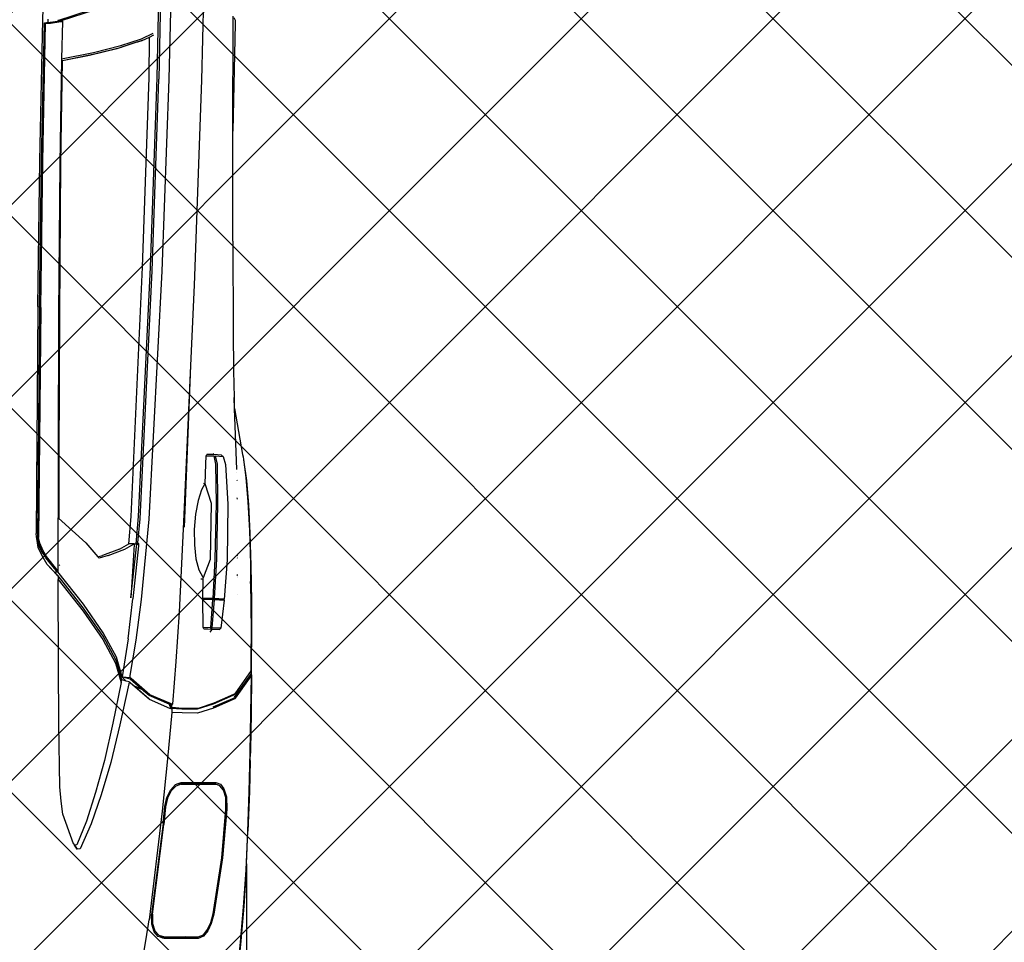
# Model space of a CAD drawing. Units: inches. Extents: x 2167 to 2589, y 1680 to 2489.
# Tile 10 of 38: x 2299 to 2335, y 1727 to 1761. Entities that reach past the tile are written whole.
import ezdxf

# ---------------------------------------------------------------- set-up
doc = ezdxf.new("R2010")
doc.units = ezdxf.units.IN
doc.header["$MEASUREMENT"] = 0
doc.layers.get('0').update_dxf_attribs({"color": 250})
doc.layers.add('C-PRKG-VEHS', color=8, linetype='Continuous', lineweight=13)
doc.layers.add('L-PVMT-PATT', color=252, linetype='Continuous', lineweight=13)
doc.layers.add('Edges', color=250, linetype='Continuous')

# ---------------------------------------------------------------- blocks, each defined once
blk = doc.blocks.new('Nissan Qashqai pl')
at = {"layer": 'Edges'}
for p, q in [((10.4926, 12.8125), (10.5294, 12.8143)), ((10.526, 12.8138), (10.569, 12.8151)), ((10.5294, 12.8143), (10.5719, 12.8156)), ((10.569, 12.8151), (10.5919, 12.8155)), ((10.5719, 12.8156), (10.6176, 12.8164)), ((10.5919, 12.8155), (10.6151, 12.8159)), ((10.5981, 12.8157), (10.5919, 12.8155)), ((10.6174, 12.816), (10.5981, 12.8157)), ((10.6151, 12.8159), (10.6644, 12.8162)), ((10.6176, 12.8164), (10.6651, 12.8167)), ((10.6644, 12.8162), (10.7078, 12.8159)), ((10.6651, 12.8167), (10.666, 12.8167)), ((10.666, 12.8167), (10.677, 12.8167)), ((10.6729, 12.8157), (10.7082, 12.8156)), ((10.6809, 12.8167), (10.677, 12.8167)), ((10.7128, 12.8166), (10.6809, 12.8167)), ((10.7078, 12.8159), (10.7083, 12.8156)), ((10.7082, 12.8156), (10.7078, 12.8159)), ((10.7085, 12.8153), (10.7082, 12.8156)), ((10.7082, 12.8156), (10.7083, 12.8156)), ((10.7083, 12.8156), (10.7087, 12.8153)), ((10.7083, 12.8156), (10.7125, 12.8156)), ((10.7087, 12.8153), (10.7363, 12.7959)), ((10.7139, 12.8164), (10.7125, 12.8156)), ((10.7137, 12.8148), (10.7125, 12.8156)), ((10.7128, 12.8166), (10.7625, 12.8161)), ((10.7128, 12.8166), (10.724, 12.8166)), ((10.7137, 12.8148), (10.7138, 12.8147)), ((10.7418, 12.7947), (10.7138, 12.8147)), ((10.7139, 12.8164), (10.7148, 12.8157)), ((10.7628, 12.8158), (10.7139, 12.8164)), ((10.7148, 12.8157), (10.7429, 12.7956)), ((10.7685, 12.8161), (10.724, 12.8166)), ((10.7625, 12.8161), (10.7628, 12.8161)), ((10.7628, 12.8161), (10.8099, 12.8152)), ((10.8131, 12.8149), (10.7628, 12.8158)), ((10.7688, 12.8161), (10.7685, 12.8161)), ((10.8099, 12.8152), (10.7688, 12.8161)), ((10.8099, 12.8152), (10.8131, 12.8152)), ((10.8134, 12.8152), (10.8131, 12.8152)), ((10.8644, 12.8135), (10.8131, 12.8149)), ((10.8134, 12.8152), (10.8142, 12.8152)), ((10.8142, 12.8152), (10.8142, 12.8152)), ((10.8237, 12.8149), (10.8142, 12.8152)), ((10.8237, 12.8149), (10.864, 12.8138)), ((10.3679, 12.7944), (10.4275, 12.8051)), ((10.4275, 12.8051), (10.4304, 12.8056)), ((10.4304, 12.8056), (10.4339, 12.8061)), ((10.4339, 12.8061), (10.4573, 12.8093)), ((10.4339, 12.8061), (10.4345, 12.8062)), ((10.4345, 12.8062), (10.4613, 12.8099)), ((10.4573, 12.8093), (10.4889, 12.8119)), ((10.4613, 12.8099), (10.4926, 12.8125)), ((10.4889, 12.8119), (10.526, 12.8138)), ((10.8596, 12.8138), (10.8589, 12.8138)), ((10.8642, 12.8136), (10.8596, 12.8138)), ((10.864, 12.8138), (10.8642, 12.8138)), ((10.8642, 12.8138), (10.9152, 12.812)), ((10.9158, 12.8118), (10.8644, 12.8135)), ((10.9577, 12.8101), (10.9152, 12.812)), ((10.9657, 12.8095), (10.9158, 12.8118)), ((10.9577, 12.8101), (10.9649, 12.8097)), ((10.9577, 12.8101), (11.1283, 12.8101)), ((10.9649, 12.8097), (11.0127, 12.8067)), ((11.0138, 12.8064), (10.9657, 12.8095)), ((11.0127, 12.8067), (11.0576, 12.8026)), ((11.059, 12.8023), (11.0138, 12.8064)), ((11.0576, 12.8026), (11.0798, 12.8008)), ((11.0768, 12.8008), (11.059, 12.8023)), ((9.8643, 12.7927), (9.8598, 12.7928)), ((9.8614, 12.7937), (9.8647, 12.7956)), ((10.0085, 12.7922), (9.8643, 12.7927)), ((9.8647, 12.7956), (9.869, 12.7954)), ((9.869, 12.7954), (10.0085, 12.7922)), ((10.0124, 12.7922), (10.0085, 12.7922)), ((10.1513, 12.7924), (10.0124, 12.7922)), ((10.1513, 12.7924), (10.2677, 12.793)), ((10.2677, 12.793), (10.3189, 12.7931)), ((10.3189, 12.7931), (10.3537, 12.7939)), ((10.3537, 12.7939), (10.3832, 12.7945)), ((10.3679, 12.7944), (10.3537, 12.7939)), ((10.4468, 12.7976), (10.3679, 12.7944)), ((10.4503, 12.7976), (10.4502, 12.7976)), ((10.4603, 12.7976), (10.4613, 12.7978)), ((10.4838, 12.7977), (10.4852, 12.7982)), ((10.5565, 12.7985), (10.5591, 12.7977)), ((10.5615, 12.7978), (10.5617, 12.7985)), ((10.583, 12.7984), (10.5834, 12.798)), ((10.5836, 12.798), (10.5831, 12.7984)), ((10.5847, 12.798), (10.5841, 12.7984)), ((10.5873, 12.7981), (10.5873, 12.7981)), ((10.6087, 12.7983), (10.6087, 12.7984)), ((10.7363, 12.7959), (10.7376, 12.795)), ((10.7387, 12.794), (10.7376, 12.795)), ((10.7376, 12.795), (10.7378, 12.7946)), ((10.7378, 12.7946), (10.7379, 12.7945)), ((10.7378, 12.7946), (10.7385, 12.7932)), ((10.7385, 12.7932), (10.7497, 12.7679)), ((10.7387, 12.794), (10.7396, 12.7922)), ((10.7396, 12.7922), (10.7507, 12.7669)), ((10.743, 12.7939), (10.7418, 12.7947)), ((10.7432, 12.7954), (10.7426, 12.7954)), ((10.7429, 12.7956), (10.7432, 12.7954)), ((10.7434, 12.793), (10.743, 12.7939)), ((10.7441, 12.7954), (10.7432, 12.7954)), ((10.7432, 12.7954), (10.744, 12.7948)), ((10.7437, 12.7921), (10.7434, 12.793)), ((10.7438, 12.7921), (10.7437, 12.7921)), ((10.7438, 12.7921), (10.7549, 12.7666)), ((10.744, 12.7948), (10.7448, 12.793)), ((10.7448, 12.793), (10.7559, 12.7674)), ((10.4282, 12.7775), (10.4274, 12.7679)), ((10.4282, 12.7775), (10.4299, 12.7798)), ((10.4291, 12.77), (10.4299, 12.7798)), ((10.4299, 12.7798), (10.4406, 12.7829)), ((10.4406, 12.7829), (10.4919, 12.7858)), ((10.4919, 12.7858), (10.564, 12.7851)), ((10.564, 12.7851), (10.6151, 12.7813)), ((10.615, 12.7803), (10.6142, 12.7686)), ((10.6151, 12.7813), (10.615, 12.7803)), ((10.615, 12.7676), (10.6151, 12.7803)), ((10.6151, 12.7803), (10.615, 12.7803)), ((10.6151, 12.7803), (10.6151, 12.7813)), ((10.6151, 12.7685), (10.616, 12.7812)), ((10.616, 12.7812), (10.6526, 12.7768)), ((10.6526, 12.7768), (10.6518, 12.7657)), ((10.6526, 12.7768), (10.6543, 12.7749)), ((10.8523, 12.7704), (10.8546, 12.7762)), ((10.8565, 12.7757), (10.8543, 12.7702)), ((10.8546, 12.7762), (10.8607, 12.7808)), ((10.8622, 12.7801), (10.8565, 12.7757)), ((10.8607, 12.7808), (10.8708, 12.7841)), ((10.8716, 12.7832), (10.8622, 12.7801)), ((10.8708, 12.7841), (10.8869, 12.7844)), ((10.887, 12.7835), (10.8716, 12.7832)), ((10.8869, 12.7844), (10.9499, 12.7789)), ((10.9498, 12.7781), (10.887, 12.7835)), ((11.0226, 12.7668), (10.9498, 12.7781)), ((10.9499, 12.7789), (11.0229, 12.7676)), ((10.4263, 12.7665), (10.4274, 12.7674)), ((10.4274, 12.7679), (10.4274, 12.7674)), ((10.4274, 12.7674), (10.4275, 12.7586)), ((10.4398, 12.7724), (10.4291, 12.77)), ((10.4291, 12.7677), (10.4398, 12.7701)), ((10.4293, 12.7579), (10.4291, 12.7677)), ((10.4909, 12.773), (10.4398, 12.7724)), ((10.4398, 12.7701), (10.4909, 12.7708)), ((10.4908, 12.7648), (10.4653, 12.7564)), ((10.563, 12.7633), (10.4908, 12.7648)), ((10.5631, 12.7715), (10.4909, 12.773)), ((10.4909, 12.7708), (10.563, 12.7692)), ((10.563, 12.7692), (10.6142, 12.7663)), ((10.5867, 12.7545), (10.563, 12.7633)), ((10.6142, 12.7686), (10.5631, 12.7715)), ((10.6142, 12.766), (10.6141, 12.7537)), ((10.6142, 12.7686), (10.6142, 12.7677)), ((10.6142, 12.7677), (10.615, 12.7676)), ((10.6142, 12.7677), (10.6142, 12.7663)), ((10.6142, 12.7663), (10.6142, 12.766)), ((10.6151, 12.7676), (10.615, 12.7676)), ((10.615, 12.7537), (10.6151, 12.7659)), ((10.6518, 12.7657), (10.6151, 12.7685)), ((10.6151, 12.7676), (10.6151, 12.7685)), ((10.6151, 12.7662), (10.6151, 12.7676)), ((10.6151, 12.7662), (10.6518, 12.7634)), ((10.6151, 12.7659), (10.6151, 12.7662)), ((10.6518, 12.7634), (10.6517, 12.754)), ((10.6536, 12.7639), (10.6518, 12.7657)), ((10.6518, 12.7657), (10.6518, 12.7634)), ((10.6518, 12.7634), (10.6536, 12.7639)), ((10.6543, 12.7656), (10.6535, 12.7546)), ((10.6535, 12.7546), (10.6536, 12.7639)), ((10.6536, 12.7639), (10.6537, 12.7658)), ((10.6537, 12.7658), (10.6543, 12.7749)), ((10.6537, 12.7658), (10.6543, 12.7656)), ((10.6543, 12.7749), (10.6543, 12.7656)), ((10.6578, 12.7628), (10.6543, 12.7656)), ((10.7497, 12.7679), (10.7565, 12.7473)), ((10.7507, 12.7669), (10.7575, 12.7462)), ((10.7559, 12.7674), (10.7626, 12.7467)), ((10.8523, 12.7255), (10.8523, 12.7704)), ((10.8543, 12.7702), (10.8538, 12.753)), ((10.8543, 12.7255), (10.8543, 12.7702)), ((11.0339, 12.7639), (11.0226, 12.7668)), ((11.0229, 12.7676), (11.0348, 12.7645)), ((11.0429, 12.7597), (11.0339, 12.7639)), ((11.0348, 12.7645), (11.0444, 12.7601)), ((9.8024, 12.7549), (9.9426, 12.7518)), ((9.9426, 12.7518), (10.2081, 12.7424)), ((10.4293, 12.7579), (10.4275, 12.7586)), ((10.4398, 12.7573), (10.4293, 12.7579)), ((10.4653, 12.7564), (10.4398, 12.7573)), ((10.4653, 12.7561), (10.4652, 12.7545)), ((10.4653, 12.7564), (10.4653, 12.7561)), ((10.4653, 12.7564), (10.4653, 12.7564)), ((10.4653, 12.7564), (10.4653, 12.7561)), ((10.4653, 12.7561), (10.4653, 12.7561)), ((10.4653, 12.7561), (10.4732, 12.7517)), ((10.4732, 12.7517), (10.4871, 12.7474)), ((10.5769, 12.7484), (10.5863, 12.7537)), ((10.5863, 12.7537), (10.5867, 12.7545)), ((10.5885, 12.7538), (10.5867, 12.7545)), ((10.5885, 12.751), (10.5885, 12.7538)), ((10.6141, 12.7537), (10.5885, 12.7538)), ((10.6141, 12.7537), (10.615, 12.7537)), ((10.6517, 12.754), (10.615, 12.7537)), ((10.6535, 12.7546), (10.6517, 12.754)), ((10.8528, 12.7503), (10.8535, 12.7521)), ((10.8528, 12.742), (10.8528, 12.7503)), ((10.8535, 12.7521), (10.8538, 12.753)), ((10.8538, 12.7521), (10.8535, 12.7521)), ((10.8538, 12.753), (10.8538, 12.7521)), ((10.8538, 12.7521), (10.8538, 12.7502)), ((10.8538, 12.7502), (10.8538, 12.742)), ((11.0497, 12.7542), (11.0429, 12.7597)), ((11.0444, 12.7601), (11.0516, 12.7542)), ((11.0523, 12.7475), (11.0497, 12.7542)), ((11.0516, 12.7542), (11.0543, 12.7473)), ((10.2081, 12.7424), (10.312, 12.7377)), ((10.312, 12.7377), (10.5214, 12.7293)), ((10.312, 12.7377), (10.5147, 12.7285)), ((10.4871, 12.7474), (10.5048, 12.744)), ((10.5048, 12.744), (10.5246, 12.7423)), ((10.5246, 12.7423), (10.5445, 12.7425)), ((10.5445, 12.7425), (10.5625, 12.7446)), ((10.5625, 12.7446), (10.5769, 12.7484)), ((10.7565, 12.7473), (10.7563, 12.7273)), ((10.7575, 12.7462), (10.7572, 12.7263)), ((10.7626, 12.7467), (10.7623, 12.7269)), ((10.8528, 12.742), (10.8538, 12.742)), ((10.8528, 12.7419), (10.8528, 12.742)), ((10.8538, 12.7419), (10.8528, 12.7419)), ((10.8528, 12.7242), (10.8528, 12.7419)), ((10.8538, 12.742), (10.8538, 12.7419)), ((10.8538, 12.7214), (10.8538, 12.7419)), ((11.0528, 12.73), (11.0523, 12.7475)), ((11.0523, 12.7312), (11.0523, 12.7475)), ((11.0543, 12.7473), (11.0543, 12.7035)), ((10.5147, 12.7285), (10.6318, 12.7228)), ((10.7563, 12.7273), (10.7553, 12.7134)), ((10.7572, 12.7263), (10.7563, 12.7126)), ((10.7623, 12.7269), (10.7615, 12.7131)), ((10.8528, 12.7242), (10.8523, 12.7255)), ((10.8543, 12.7255), (10.8569, 12.7184)), ((11.0523, 12.7312), (11.0528, 12.73)), ((11.0523, 12.7287), (11.0523, 12.7312)), ((11.0528, 12.7274), (11.0523, 12.7287)), ((11.0523, 12.7037), (11.0523, 12.7287)), ((11.0528, 12.7274), (11.0528, 12.73)), ((11.0528, 12.73), (11.0538, 12.7273)), ((11.0528, 12.7274), (11.0528, 12.6985)), ((11.0538, 12.7273), (11.0538, 12.7018)), ((9.9414, 12.71), (9.8143, 12.713)), ((10.6318, 12.7228), (10.6955, 12.7184)), ((10.6955, 12.7184), (10.7509, 12.714)), ((10.7507, 12.7132), (10.7501, 12.7114)), ((10.7506, 12.7111), (10.7507, 12.7132)), ((10.7507, 12.7132), (10.7509, 12.714)), ((10.751, 12.7132), (10.7507, 12.7132)), ((10.7522, 12.7131), (10.7509, 12.714)), ((10.7516, 12.7131), (10.7509, 12.714)), ((10.7519, 12.7128), (10.7511, 12.7107)), ((10.7522, 12.7131), (10.7516, 12.7131)), ((10.7519, 12.7128), (10.7516, 12.7131)), ((10.7526, 12.7124), (10.7519, 12.7128)), ((10.7553, 12.7134), (10.7522, 12.7131)), ((10.7524, 12.7106), (10.7526, 12.7124)), ((10.7556, 12.7122), (10.7524, 12.7106)), ((10.7526, 12.7124), (10.7526, 12.7127)), ((10.7532, 12.712), (10.7526, 12.7124)), ((10.7556, 12.7122), (10.7532, 12.712)), ((10.7561, 12.7125), (10.7556, 12.7122)), ((10.7561, 12.7125), (10.7563, 12.7126)), ((10.7563, 12.7125), (10.7561, 12.7125)), ((10.7563, 12.7123), (10.7561, 12.7123)), ((10.7563, 12.7126), (10.7573, 12.7135)), ((10.7563, 12.7126), (10.7563, 12.7125)), ((10.7569, 12.7125), (10.7563, 12.7109)), ((10.7569, 12.7125), (10.7563, 12.7125)), ((10.7563, 12.7125), (10.7563, 12.7123)), ((10.7573, 12.7135), (10.7569, 12.7125)), ((10.7573, 12.7135), (10.7604, 12.7132)), ((10.7604, 12.7132), (10.7615, 12.7131)), ((10.7615, 12.7131), (10.8218, 12.7077)), ((10.8538, 12.7214), (10.8528, 12.7242)), ((10.855, 12.7181), (10.8538, 12.7214)), ((10.8622, 12.7114), (10.855, 12.7181)), ((10.8569, 12.7184), (10.8637, 12.712)), ((10.8637, 12.712), (10.8727, 12.7077)), ((9.8101, 12.6993), (9.9411, 12.6966)), ((10.19, 12.7008), (9.9414, 12.71)), ((10.5113, 12.6839), (10.19, 12.7008)), ((10.7501, 12.7114), (10.7387, 12.6849)), ((10.7507, 12.7098), (10.7397, 12.684)), ((10.7563, 12.7109), (10.7449, 12.6843)), ((10.7511, 12.7107), (10.7507, 12.7098)), ((10.7524, 12.7106), (10.7507, 12.7098)), ((10.8218, 12.7077), (10.8896, 12.7008)), ((10.8718, 12.7068), (10.8622, 12.7114)), ((10.8836, 12.7041), (10.8718, 12.7068)), ((10.8727, 12.7077), (10.8839, 12.7051)), ((10.9054, 12.702), (10.8836, 12.7041)), ((10.8839, 12.7051), (10.9067, 12.7029)), ((10.8896, 12.7008), (11.0304, 12.6838)), ((10.9054, 12.702), (11.0232, 12.6871)), ((11.0231, 12.6882), (10.9067, 12.7029)), ((11.0501, 12.6964), (11.0523, 12.7037)), ((11.0538, 12.7018), (11.0528, 12.6985)), ((11.0543, 12.7035), (11.0538, 12.7018)), ((9.9393, 12.6944), (9.8119, 12.697)), ((9.8891, 12.6741), (9.8818, 12.6891)), ((9.8867, 12.6842), (9.8838, 12.6901)), ((10.1849, 12.6857), (9.9393, 12.6944)), ((10.1894, 12.6879), (9.9411, 12.6966)), ((10.5109, 12.6721), (10.1894, 12.6879)), ((11.0231, 12.6882), (11.035, 12.6883)), ((11.0358, 12.6872), (11.0232, 12.6871)), ((11.035, 12.6883), (11.0443, 12.6911)), ((11.0458, 12.6903), (11.0358, 12.6872)), ((11.0443, 12.6911), (11.0501, 12.6964)), ((11.052, 12.6958), (11.0458, 12.6903)), ((11.0528, 12.6985), (11.052, 12.6958)), ((9.9393, 12.684), (9.8867, 12.6842)), ((9.8911, 12.675), (9.8867, 12.6842)), ((9.8978, 12.6472), (9.8891, 12.6741)), ((9.8911, 12.6749), (9.8911, 12.675)), ((9.8931, 12.6691), (9.8911, 12.6749)), ((9.8911, 12.6749), (9.8998, 12.6481)), ((10.1849, 12.6754), (9.9393, 12.684)), ((10.5079, 12.6703), (10.1849, 12.6857)), ((10.5079, 12.6607), (10.1849, 12.6754)), ((10.6152, 12.674), (10.5113, 12.6839)), ((10.6678, 12.6672), (10.6152, 12.674)), ((10.7387, 12.6849), (10.7177, 12.6604)), ((10.7334, 12.6766), (10.7186, 12.6593)), ((10.7449, 12.6843), (10.7232, 12.6594)), ((10.7438, 12.6836), (10.7265, 12.6635)), ((10.7265, 12.6635), (10.7316, 12.6741)), ((10.7397, 12.684), (10.7334, 12.6766)), ((11.0357, 12.6829), (11.0304, 12.6838)), ((11.0491, 12.6807), (11.0357, 12.6829)), ((11.0449, 12.6812), (11.0448, 12.6812)), ((11.0492, 12.6807), (11.0491, 12.6807)), ((11.1336, 12.667), (11.0492, 12.6807)), ((9.8931, 12.669), (9.8931, 12.6691)), ((9.8931, 12.669), (9.9018, 12.6421)), ((10.543, 12.6671), (10.5079, 12.6703)), ((10.5417, 12.6693), (10.5109, 12.6721)), ((10.5417, 12.6693), (10.5427, 12.6702)), ((10.5417, 12.6693), (10.543, 12.6671)), ((10.5436, 12.6687), (10.5427, 12.6702)), ((10.5427, 12.6702), (10.5458, 12.67)), ((10.544, 12.6678), (10.543, 12.6671)), ((10.543, 12.6646), (10.543, 12.6671)), ((10.543, 12.6646), (10.543, 12.6576)), ((10.5439, 12.6646), (10.543, 12.6646)), ((10.5502, 12.6526), (10.543, 12.6646)), ((10.544, 12.6678), (10.5436, 12.6687)), ((10.5439, 12.6646), (10.613, 12.6601)), ((10.547, 12.6674), (10.544, 12.6678)), ((10.5458, 12.67), (10.6144, 12.6629)), ((10.613, 12.6601), (10.547, 12.6674)), ((10.6664, 12.6566), (10.6144, 12.6629)), ((10.7137, 12.6595), (10.6678, 12.6672)), ((10.7265, 12.6635), (10.7224, 12.6587)), ((9.9086, 12.6129), (9.8998, 12.6481)), ((10.543, 12.6576), (10.5079, 12.6607)), ((10.5502, 12.6456), (10.543, 12.6576)), ((10.5584, 12.6306), (10.5502, 12.6526)), ((10.6664, 12.6566), (10.7155, 12.649)), ((10.7155, 12.649), (10.69, 12.6414)), ((10.7165, 12.6591), (10.7137, 12.6595)), ((10.7186, 12.6593), (10.7155, 12.649)), ((10.7155, 12.649), (10.7165, 12.6591)), ((10.7209, 12.654), (10.7155, 12.6485)), ((10.7155, 12.649), (10.7155, 12.6485)), ((10.7155, 12.6485), (10.7155, 12.6473)), ((10.7192, 12.6484), (10.7155, 12.6473)), ((10.7177, 12.6604), (10.7165, 12.6591)), ((10.7209, 12.654), (10.7192, 12.6484)), ((10.7228, 12.6477), (10.7192, 12.6484)), ((10.7221, 12.6581), (10.7209, 12.654)), ((10.7232, 12.6594), (10.7221, 12.6581)), ((10.7221, 12.6581), (10.7224, 12.6587)), ((10.7221, 12.6581), (10.7247, 12.6575)), ((10.7247, 12.6575), (10.7776, 12.646)), ((9.9066, 12.6119), (9.8978, 12.6472)), ((9.9018, 12.6421), (9.9106, 12.6068)), ((10.5502, 12.6456), (10.5584, 12.6236)), ((10.69, 12.6414), (10.6583, 12.6245)), ((10.6943, 12.641), (10.6627, 12.6241)), ((10.6671, 12.6238), (10.6976, 12.6401)), ((10.7155, 12.6473), (10.6943, 12.641)), ((10.6976, 12.6401), (10.7228, 12.6477)), ((10.7228, 12.6477), (10.7754, 12.637)), ((10.7754, 12.637), (10.8239, 12.6261)), ((10.7776, 12.646), (10.8264, 12.6341)), ((10.5584, 12.6306), (10.5617, 12.619)), ((10.56, 12.6176), (10.5584, 12.6236)), ((10.6583, 12.6245), (10.6215, 12.5986)), ((10.6627, 12.6241), (10.6261, 12.5984)), ((10.6306, 12.5982), (10.6671, 12.6238)), ((10.8239, 12.6261), (10.8653, 12.6144)), ((10.8264, 12.6341), (10.8682, 12.6216)), ((9.8652, 12.5704), (9.8516, 12.6129)), ((9.9149, 12.5705), (9.9066, 12.6119)), ((9.9169, 12.5714), (9.9086, 12.6129)), ((10.5419, 12.6018), (10.56, 12.6176)), ((10.56, 12.6176), (10.5617, 12.619)), ((10.8653, 12.6144), (10.9026, 12.6025)), ((10.8682, 12.6216), (10.9059, 12.6087)), ((9.8652, 12.5654), (9.8516, 12.6079)), ((9.9106, 12.6068), (9.9177, 12.5714)), ((10.51, 12.5666), (10.5419, 12.6018)), ((10.6215, 12.5986), (10.5796, 12.5655)), ((10.5892, 12.5659), (10.6306, 12.5982)), ((10.6261, 12.5984), (10.593, 12.5726)), ((10.9026, 12.6025), (10.933, 12.5901)), ((10.9059, 12.6087), (10.9384, 12.5945)), ((10.9316, 12.586), (10.8932, 12.572)), ((10.9316, 12.586), (10.9334, 12.5872)), ((10.932, 12.5862), (10.9316, 12.586)), ((10.9335, 12.5871), (10.932, 12.5862)), ((10.933, 12.5901), (10.9334, 12.5872)), ((10.9334, 12.5872), (10.9386, 12.5905)), ((10.9334, 12.5872), (10.9335, 12.5871)), ((10.9386, 12.5905), (10.9335, 12.5871)), ((10.9384, 12.5945), (10.9386, 12.5905)), ((10.593, 12.5726), (10.584, 12.5655)), ((10.8932, 12.572), (10.8766, 12.5697)), ((9.8652, 12.5706), (9.8664, 12.5714)), ((9.8652, 12.5706), (9.8665, 12.5695)), ((9.8652, 12.5704), (9.8652, 12.5706)), ((9.8652, 12.5704), (9.8652, 12.5704)), ((9.8652, 12.5704), (9.8652, 12.5654)), ((9.8655, 12.5687), (9.8652, 12.5704)), ((9.8675, 12.5555), (9.8655, 12.5687)), ((9.8665, 12.5695), (9.8664, 12.5714)), ((9.8664, 12.5714), (9.9149, 12.5705)), ((9.8686, 12.5562), (9.8665, 12.5695)), ((9.9149, 12.5705), (10.0505, 12.5681)), ((9.9177, 12.5714), (9.9169, 12.5714)), ((10.0501, 12.5695), (9.9177, 12.5714)), ((10.2453, 12.568), (10.0501, 12.5695)), ((10.0505, 12.5681), (10.2453, 12.5664)), ((10.4292, 12.5674), (10.2453, 12.568)), ((10.2453, 12.5664), (10.4289, 12.5658)), ((10.4289, 12.5658), (10.5092, 12.5658)), ((10.5099, 12.5674), (10.4292, 12.5674)), ((10.5099, 12.5674), (10.5092, 12.5658)), ((10.5092, 12.5658), (10.5094, 12.5658)), ((10.5094, 12.5658), (10.51, 12.5666)), ((10.5783, 12.5659), (10.5094, 12.5658)), ((10.51, 12.5666), (10.5099, 12.5674)), ((10.5764, 12.5642), (10.5598, 12.5507)), ((10.5776, 12.5633), (10.5612, 12.5498)), ((10.5834, 12.5641), (10.57, 12.5517)), ((10.57, 12.5517), (10.5821, 12.5633)), ((10.5709, 12.5675), (10.5705, 12.5671)), ((10.5719, 12.5682), (10.5709, 12.5675)), ((10.5783, 12.5659), (10.5764, 12.5642)), ((10.5776, 12.5633), (10.5783, 12.5659)), ((10.5796, 12.5655), (10.5776, 12.5633)), ((10.5796, 12.5655), (10.5783, 12.5659)), ((10.5796, 12.562), (10.5796, 12.5655)), ((10.5838, 12.5653), (10.5821, 12.5633)), ((10.584, 12.5647), (10.5834, 12.5641)), ((10.584, 12.5655), (10.5838, 12.5653)), ((10.584, 12.5655), (10.5841, 12.5655)), ((10.584, 12.5654), (10.584, 12.5655)), ((10.5847, 12.5655), (10.584, 12.5647)), ((10.584, 12.5647), (10.584, 12.5654)), ((10.5851, 12.5659), (10.5841, 12.5655)), ((10.5841, 12.5655), (10.5847, 12.5655)), ((10.5851, 12.5659), (10.5847, 12.5655)), ((10.5851, 12.5659), (10.5892, 12.5659)), ((10.6988, 12.5662), (10.5892, 12.5659)), ((10.7769, 12.5667), (10.6988, 12.5662)), ((10.858, 12.5683), (10.7769, 12.5667)), ((10.8766, 12.5697), (10.858, 12.5683)), ((9.8644, 12.5459), (9.696, 12.551)), ((9.8643, 12.5532), (9.8637, 12.5532)), ((9.8677, 12.5531), (9.8643, 12.5532)), ((10.0472, 12.5423), (9.8644, 12.5459)), ((9.8677, 12.5531), (9.8675, 12.5555)), ((9.8678, 12.5507), (9.8677, 12.5531)), ((9.8681, 12.5482), (9.8678, 12.5507)), ((9.8681, 12.5482), (9.869, 12.5496)), ((10.0476, 12.5445), (9.8681, 12.5482)), ((9.8689, 12.5515), (9.8686, 12.5562)), ((9.869, 12.5496), (9.8689, 12.5515)), ((10.0477, 12.5459), (9.869, 12.5496)), ((10.2369, 12.5433), (10.0477, 12.5459)), ((10.5522, 12.5465), (10.5422, 12.542)), ((10.5546, 12.546), (10.5495, 12.5438)), ((10.5598, 12.5507), (10.5522, 12.5465)), ((10.5583, 12.5481), (10.5546, 12.546)), ((10.5551, 12.5457), (10.5583, 12.5481)), ((10.5612, 12.5498), (10.5583, 12.5481)), ((10.57, 12.5517), (10.5589, 12.5451)), ((10.2357, 12.5398), (10.0472, 12.5423)), ((10.2367, 12.5419), (10.0476, 12.5445)), ((10.2357, 12.5398), (10.53, 12.5373)), ((10.2367, 12.5419), (10.5351, 12.5392)), ((10.2369, 12.5433), (10.5348, 12.5406)), ((10.4153, 12.5384), (10.4176, 12.5384)), ((10.4176, 12.5384), (10.4181, 12.5384)), ((10.4181, 12.5384), (10.4552, 12.538)), ((10.4181, 12.5384), (10.4181, 12.5384)), ((10.4778, 12.5378), (10.53, 12.5373)), ((10.5301, 12.5373), (10.53, 12.5373)), ((10.5335, 12.5378), (10.5301, 12.5373)), ((10.5419, 12.5391), (10.5335, 12.5378)), ((10.5422, 12.542), (10.5348, 12.5406)), ((10.5418, 12.5405), (10.5351, 12.5392)), ((10.5424, 12.5406), (10.5418, 12.5405)), ((10.5419, 12.5391), (10.5463, 12.541)), ((10.5479, 12.54), (10.5419, 12.5391)), ((10.5495, 12.5438), (10.5424, 12.5406)), ((10.5463, 12.541), (10.5551, 12.5457)), ((10.5589, 12.5451), (10.5479, 12.54))]:
    blk.add_line(p, q, dxfattribs=at)
blk = doc.blocks.new('car')
blk.add_blockref('Nissan Qashqai pl', (-9.7433, -11.9151))
blk = doc.blocks.new('carr')
blk.add_blockref('car', (0.5124, -0.007))

msp = doc.modelspace()

# ---------------------------------------------------------------- hatches: boundary and pattern name
at = {"layer": 'L-PVMT-PATT'}
h = msp.add_hatch(dxfattribs=at)
h.set_pattern_fill('ANSI37', color=256, scale=40)
h.paths.add_polyline_path([(2417.548, 1783.695), (2417.548, 1846.042), (2239.361, 1846.042), (2239.361, 1687.695), (2369.843, 1687.695), (2369.843, 1696.695), (2375.607, 1696.695), (2416.107, 1696.695), (2417.548, 1696.695)])

# ---------------------------------------------------------------- block references
at = {"layer": 'C-PRKG-VEHS', "xscale": 28.42784210623918, "yscale": 28.42784210623918, "zscale": 28.42784210623918, "rotation": 270}
msp.add_blockref('carr', (2281.736, 1778.659), dxfattribs=at)

doc.saveas('drawing.dxf')
